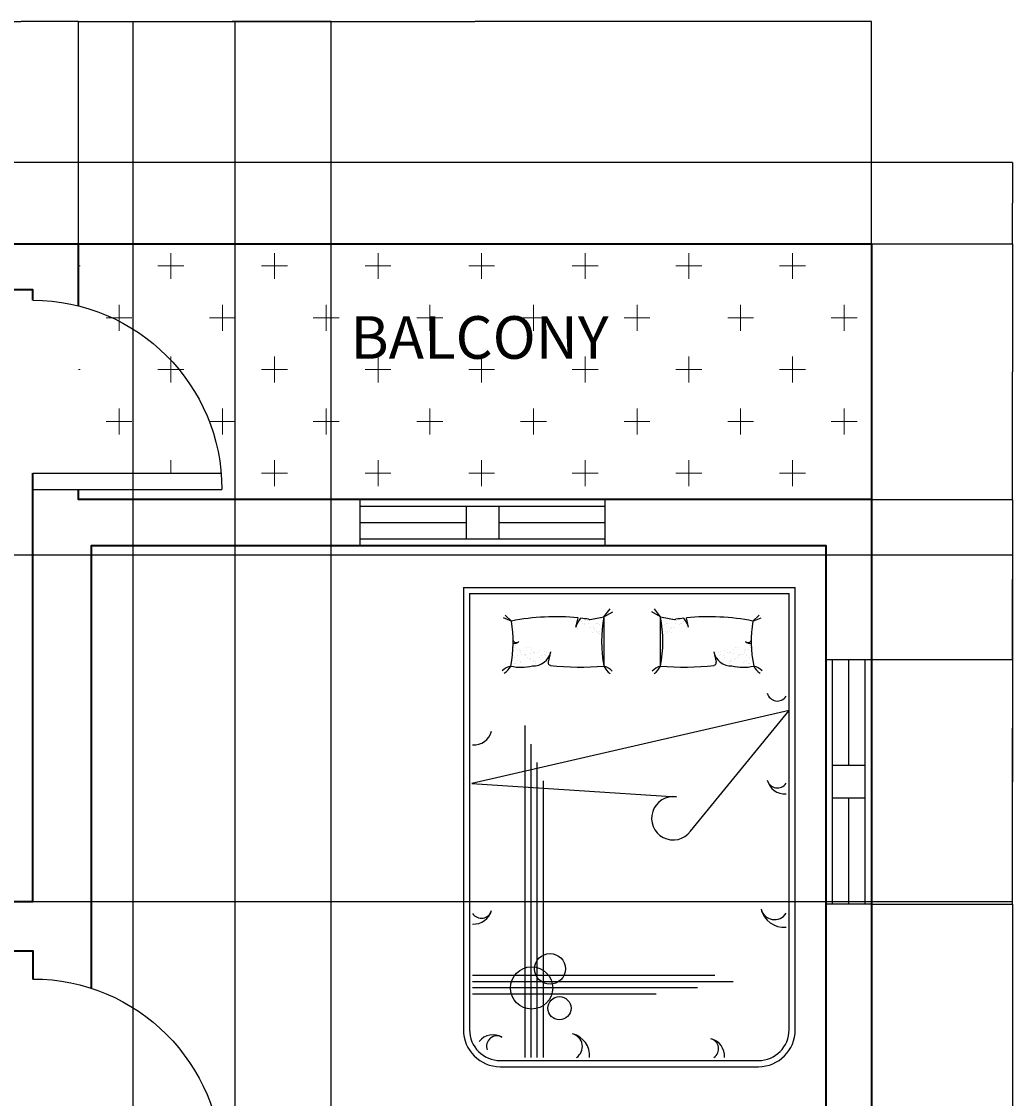
# Model space of a CAD drawing. Units: millimetres. Extents: x 19292 to 100733, y 12374 to 26974.
# Tile 22 of 24: x 52672 to 57530, y 18270 to 23551. Entities that reach past the tile are written whole.
import ezdxf

# ---------------------------------------------------------------- set-up
doc = ezdxf.new("R2010")
doc.units = ezdxf.units.MM
for name, color, linetype, lineweight in [('A-ANNO-DIMS', 2, 'Continuous', 18), ('A-AREA-IDEN', 3, 'Continuous', 25), ('A-DOOR', 4, 'Continuous', 25), ('A-FLOR-PATT', 252, 'Continuous', 13), ('A-FURN', 8, 'Continuous', 18), ('A-GLAZ', 3, 'Continuous', 25), ('A-WALL', 7, 'Continuous', 35)]:
    doc.layers.add(name, color=color, linetype=linetype, lineweight=lineweight)
doc.layers.add('FURNITURE', color=40, linetype='Continuous')
doc.layers.add('WINDOWS', color=50, linetype='Continuous')
doc.styles.get("Standard").update_dxf_attribs({"font": 'arial.ttf'})
doc.dimstyles.get("Standard").update_dxf_attribs({"dimtxt": 0.18, "dimasz": 0.18, "dimexe": 0.18, "dimexo": 0.0625, "dimgap": 0.09, "dimtad": 0, "dimtih": 1, "dimtoh": 1, "dimdec": 4, "dimzin": 0, "dimdsep": 46, "dimtxsty": 'Standard', "dimcen": 0.09, "dimadec": 0, "dimazin": 0, "dimtfac": 1, "dimtdec": 4, "dimtofl": 0, "dimtmove": 0, "dimatfit": 3, "dimfxl": 1, "dimtolj": 1, "dimtzin": 0, "dimarcsym": 0})

# ---------------------------------------------------------------- blocks, each defined once
blk = doc.blocks.new('WW')
at = {"layer": 'WINDOWS'}
for p, q in [((-5183.9, -4940.9), (-3983.9, -4940.9)), ((-4663.9, -4940.9), (-4663.9, -5100.9)), ((-4503.9, -4940.9), (-4503.9, -5100.9)), ((-4503.9, -4940.9), (-4503.9, -5100.9)), ((-5183.9, -5020.9), (-4663.9, -5020.9)), ((-4503.9, -5020.9), (-3983.9, -5020.9)), ((-5183.9, -5100.9), (-3983.9, -5100.9))]:
    blk.add_line(p, q, dxfattribs=at)
for points in [[(-5183.9, -5133.4), (-5183.9, -4908.4)], [(-3983.9, -4908.4), (-3983.9, -5133.4)]]:
    blk.add_lwpolyline(points, dxfattribs=at)
blk = doc.blocks.new('DBED-4FT6')
at = {"layer": 'FURNITURE'}
for p, q in [((-27, 0), (-27, -72)), ((-27, 0), (27, 0)), ((27, -72), (27, 0)), ((-26, -1), (-26, -72)), ((-26, -1), (26, -1)), ((26, -72), (26, -1)), ((-4.13, -4.82), (-3.14, -3.5)), ((5.06, -4.82), (4.07, -3.5)), ((-19.18, -5.49), (-20.5, -4.97)), ((-19.18, -5.49), (-20.21, -4.5)), ((-8.71, -6.49), (-8.35, -4.95)), ((-7.52, -5.09), (-7.52, -5.09)), ((-7.37, -5.22), (-7.37, -5.22)), ((-5.67, -5.22), (-5.67, -5.22)), ((-4.58, -5.08), (-4.58, -5.08)), ((-4.25, -5.03), (-4.25, -5.03)), ((-4.13, -4.82), (-2.71, -4)), ((5.06, -4.82), (3.64, -4)), ((5.18, -5.03), (5.18, -5.03)), ((5.51, -5.08), (5.51, -5.08)), ((6.6, -5.22), (6.6, -5.22)), ((8.29, -5.22), (8.29, -5.22)), ((8.44, -5.09), (8.44, -5.09)), ((9.64, -6.49), (9.28, -4.95)), ((20.11, -5.49), (21.13, -4.5)), ((20.11, -5.49), (21.43, -4.97)), ((-8.41, -6.64), (-8.41, -6.64)), ((-8.24, -5.56), (-8.24, -5.56)), ((-7.82, -5.51), (-7.82, -5.51)), ((-7.61, -5.81), (-7.61, -5.81)), ((-7.37, -5.85), (-7.37, -5.85)), ((-7.27, -6.02), (-7.27, -6.02)), ((-6.74, -5.36), (-6.74, -5.36)), ((-6.57, -5.95), (-6.57, -5.95)), ((-6.25, -6.56), (-6.25, -6.56)), ((-6.09, -5.28), (-6.09, -5.28)), ((-5.88, -6.59), (-5.88, -6.59)), ((-5.73, -6.73), (-5.73, -6.73)), ((-5.28, -5.82), (-5.28, -5.82)), ((-5.12, -5.81), (-5.12, -5.81)), ((-4.78, -6.02), (-4.78, -6.02)), ((5.71, -6.02), (5.71, -6.02)), ((6.05, -5.81), (6.05, -5.81)), ((6.21, -5.82), (6.21, -5.82)), ((6.65, -6.73), (6.65, -6.73)), ((6.8, -6.59), (6.8, -6.59)), ((7.01, -5.28), (7.01, -5.28)), ((7.17, -6.56), (7.17, -6.56)), ((7.5, -5.95), (7.5, -5.95)), ((7.66, -5.36), (7.66, -5.36)), ((8.2, -6.02), (8.2, -6.02)), ((8.3, -5.85), (8.3, -5.85)), ((8.54, -5.81), (8.54, -5.81)), ((8.75, -5.51), (8.75, -5.51)), ((9.17, -5.56), (9.17, -5.56)), ((9.33, -6.64), (9.33, -6.64)), ((-6, -7.34), (-6, -7.34)), ((-5.69, -7.03), (-5.69, -7.03)), ((-5.35, -7.25), (-5.35, -7.25)), ((-5.23, -7.36), (-5.23, -7.36)), ((-4.93, -7.2), (-4.93, -7.2)), ((-4.93, -7.46), (-4.93, -7.46)), ((5.86, -7.2), (5.86, -7.2)), ((5.86, -7.46), (5.86, -7.46)), ((6.16, -7.36), (6.16, -7.36)), ((6.27, -7.25), (6.27, -7.25)), ((6.61, -7.03), (6.61, -7.03)), ((6.92, -7.34), (6.92, -7.34)), ((-18.78, -9.84), (-18.78, -9.84)), ((-18.75, -9.83), (-18.75, -9.83)), ((-18.6, -9.46), (-18.6, -9.46)), ((-18.44, -10.05), (-18.44, -10.05)), ((-17.9, -10.1), (-17.9, -10.1)), ((-17.75, -10.24), (-17.75, -10.24)), ((-16.7, -9.84), (-16.7, -9.84)), ((-16.28, -9.83), (-16.28, -9.83)), ((-15.95, -10.05), (-15.95, -10.05)), ((-14.55, -10.26), (-14.55, -10.26)), ((-13.87, -10.45), (-13.87, -10.45)), ((-12.81, -10.5), (-13.21, -12.2)), ((13.73, -10.5), (14.13, -12.2)), ((14.8, -10.45), (14.8, -10.45)), ((15.48, -10.26), (15.48, -10.26)), ((16.87, -10.05), (16.87, -10.05)), ((17.21, -9.83), (17.21, -9.83)), ((17.63, -9.84), (17.63, -9.84)), ((18.68, -10.24), (18.68, -10.24)), ((18.83, -10.1), (18.83, -10.1)), ((19.36, -10.05), (19.36, -10.05)), ((19.52, -9.46), (19.52, -9.46)), ((19.67, -9.83), (19.67, -9.83)), ((19.7, -9.84), (19.7, -9.84)), ((-18.7, -11.37), (-18.7, -11.37)), ((-18.18, -11.01), (-18.18, -11.01)), ((-18.13, -11.84), (-18.13, -11.84)), ((-17.79, -12.06), (-17.79, -12.06)), ((-17.73, -10.63), (-17.73, -10.63)), ((-17.68, -12.17), (-17.68, -12.17)), ((-17.53, -10.93), (-17.53, -10.93)), ((-17.11, -10.87), (-17.11, -10.87)), ((-16.96, -10.97), (-16.96, -10.97)), ((-16.85, -11.06), (-16.85, -11.06)), ((-16.65, -11.38), (-16.65, -11.38)), ((-16.26, -11.6), (-16.26, -11.6)), ((-16.11, -11.74), (-16.11, -11.74)), ((-16.03, -10.73), (-16.03, -10.73)), ((-15.64, -11.84), (-15.64, -11.84)), ((-15.57, -10.56), (-15.57, -10.56)), ((-15.52, -12.1), (-15.52, -12.1)), ((-15.38, -10.64), (-15.38, -10.64)), ((-15.3, -12.05), (-15.3, -12.05)), ((-14.96, -10.59), (-14.96, -10.59)), ((-14.56, -11.36), (-14.56, -11.36)), ((-14.36, -11.06), (-14.36, -11.06)), ((-13.86, -10.9), (-13.86, -10.9)), ((-13.71, -11.04), (-13.71, -11.04)), ((-13.52, -10.57), (-13.52, -10.57)), ((14.45, -10.57), (14.45, -10.57)), ((14.63, -11.04), (14.63, -11.04)), ((14.78, -10.9), (14.78, -10.9)), ((15.29, -11.06), (15.29, -11.06)), ((15.48, -11.36), (15.48, -11.36)), ((15.89, -10.59), (15.89, -10.59)), ((16.23, -12.05), (16.23, -12.05)), ((16.3, -10.64), (16.3, -10.64)), ((16.45, -12.1), (16.45, -12.1)), ((16.5, -10.56), (16.5, -10.56)), ((16.56, -11.84), (16.56, -11.84)), ((16.95, -10.73), (16.95, -10.73)), ((17.04, -11.74), (17.04, -11.74)), ((17.19, -11.6), (17.19, -11.6)), ((17.58, -11.38), (17.58, -11.38)), ((17.78, -11.06), (17.78, -11.06)), ((17.88, -10.97), (17.88, -10.97)), ((18.04, -10.87), (18.04, -10.87)), ((18.46, -10.93), (18.46, -10.93)), ((18.61, -12.17), (18.61, -12.17)), ((18.66, -10.63), (18.66, -10.63)), ((18.72, -12.06), (18.72, -12.06)), ((19.06, -11.84), (19.06, -11.84)), ((19.11, -11.01), (19.11, -11.01)), ((19.62, -11.37), (19.62, -11.37)), ((-18.67, -12.31), (-18.67, -12.31)), ((-18.65, -12.91), (-18.65, -12.91)), ((-18.52, -12.44), (-18.52, -12.44)), ((-17.44, -12.99), (-17.44, -12.99)), ((-16.79, -12.9), (-16.79, -12.9)), ((-16.6, -12.92), (-16.6, -12.92)), ((-16.38, -12.85), (-16.38, -12.85)), ((-15.32, -12.47), (-15.32, -12.47)), ((-15.29, -12.7), (-15.29, -12.7)), ((16.22, -12.7), (16.22, -12.7)), ((16.24, -12.47), (16.24, -12.47)), ((17.3, -12.85), (17.3, -12.85)), ((17.53, -12.92), (17.53, -12.92)), ((17.72, -12.9), (17.72, -12.9)), ((18.37, -12.99), (18.37, -12.99)), ((19.44, -12.44), (19.44, -12.44)), ((19.57, -12.91), (19.57, -12.91)), ((19.59, -12.31), (19.59, -12.31)), ((26, -20.04), (-25.63, -31.9)), ((9.97, -39.68), (26, -20.04)), ((-16.98, -76.5), (-16.98, -22.5)), ((-15.98, -76.5), (-15.98, -25.5)), ((-14.98, -76.5), (-14.98, -28.5)), ((-13.98, -76.5), (-13.98, -31.5)), ((-25.63, -31.9), (7.69, -34.11)), ((13.92, -63.19), (-25.5, -63.19)), ((16.88, -64.19), (-25.5, -64.19)), ((11.1, -65.19), (-25.5, -65.19)), ((4.38, -66.19), (-25.5, -66.19)), ((-21, -77), (21, -77)), ((-21, -78), (21, -78))]:
    blk.add_line(p, q, dxfattribs=at)
for centre, radius in [((-12.91, -62.08), 2.5), ((-15.91, -65.19), 3.44), ((-11.37, -68.48), 1.88)]:
    blk.add_circle(centre, radius, dxfattribs=at)
for centre, radius, start, end in [((-11.96, -41.82), 37.04, 84.4029, 101.2371), ((-4.83, -7.61), 4.05, 139.9098, 163.9756), ((-11.52, -33.35), 28.57, 80.1409, 82.7554), ((-6.49, -4.41), 0.8, 260.1409, 276.0318), ((-67.64, 360.61), 370.91, 279.5022, 279.8589), ((15.67, -8.82), 20.2, 168.5788, 191.4212), ((15.67, -8.82), 20.2, 168.5788, 191.4212), ((42751.26, -8.82), 42755.4, 179.99464, 180.00536), ((-14.74, -8.82), 20.2, 348.5788, 11.4212), ((-42750.34, -8.82), 42755.4, 359.99464, 0.00536), ((-14.74, -8.82), 20.2, 348.5788, 11.4212), ((68.57, 360.61), 370.91, 260.1411, 260.4978), ((7.42, -4.41), 0.8, 263.9682, 279.8591), ((12.45, -33.35), 28.57, 97.2446, 99.8591), ((5.75, -7.61), 4.05, 16.0244, 40.0902), ((12.89, -41.82), 37.04, 78.7629, 95.5971), ((-39.11, -8.82), 20.2, 348.607, 9.4917), ((40.03, -8.82), 20.2, 170.5083, 191.393), ((-18.4, -8.45), 0.546, 201.8041, 319.1334), ((19.33, -8.45), 0.546, 220.8666, 338.1959), ((-18.63, -8.36), 0.782, 249.4969, 325.7978), ((-15.61, -9.92), 2.87, 266.7825, 348.1719), ((16.54, -9.92), 2.87, 191.8281, 273.2175), ((19.56, -8.36), 0.782, 214.2022, 290.5031), ((-12.82, -12.29), 0.4, 166.7873, 262.877), ((13.74, -12.29), 0.4, 277.123, 13.2127), ((-18.78, -15.36), 2.61, 101.6935, 136.5635), ((-21.65, -11.66), 2.61, 299.1485, 334.0185), ((-17.6, -5.62), 7.39, 256.6499, 284.2856), ((-7.85, 31.23), 44.21, 263.4826, 274.8199), ((-1.73, -11.81), 2.61, 202.7243, 237.5943), ((-4.81, -15.34), 2.61, 40.1792, 75.0493), ((5.73, -15.34), 2.61, 104.9507, 139.8208), ((2.65, -11.81), 2.61, 302.4057, 337.2757), ((8.78, 31.23), 44.21, 265.1801, 276.5174), ((18.52, -5.62), 7.39, 255.7144, 283.3501), ((19.7, -15.36), 2.61, 43.4365, 78.3065), ((22.58, -11.66), 2.61, 205.9815, 240.8515), ((24.08, -16.81), 1.69, 194.4515, 326.9106), ((-25.29, -22.71), 2.93, 265.8594, 345.9527), ((24.08, -30.96), 1.69, 194.4515, 326.9106), ((25.29, -30.67), 2.93, 194.0473, 274.1406), ((7.14, -37.58), 3.52, 81.0159, 323.3832), ((-25.29, -51.86), 2.93, 265.8594, 345.9527), ((-24.08, -52.15), 1.69, 213.0894, 345.5485), ((23.61, -51.81), 2.26, 194.4515, 326.9106), ((25.22, -51.42), 3.91, 194.0473, 274.1406), ((-21, -72), 6, 180, 270), ((-21, -72), 5, 180, 270), ((-22.19, -75.74), 2.93, 59.0473, 140.6217), ((-21.54, -74.68), 1.69, 59.4515, 200.6983), ((-9.76, -74.73), 2.12, 303.0894, 75.5485), ((-10.12, -76.24), 3.67, 355.8594, 75.9527), ((12.55, -76.29), 2.93, 355.8594, 75.9527), ((12.84, -75.08), 1.69, 303.0894, 75.5485), ((21, -72), 5, 270, 0), ((21, -72), 6, 270, 0)]:
    blk.add_arc(centre, radius, start, end, dxfattribs=at)
blk = doc.blocks.new('DOOR-SWING-900')
blk.add_line((927.7, 927.7), (927.7, 0))
blk.add_arc((927.7, 927.7), 927.7, 180, 270)
blk = doc.blocks.new('*D98')
at = {"layer": 'A-ANNO-DIMS', "color": 0, "lineweight": -2, "transparency": 16777216}
for p, q in [((52386.5, 22460.8), (52386.5, 23550.9)), ((52386.7, 23550.7), (52668.7, 23550.7)), ((52951.3, 23550.7), (52669.3, 23550.7)), ((52951.5, 22460.8), (52951.5, 23550.9))]:
    blk.add_line(p, q, dxfattribs=at)
at = {"layer": 'A-ANNO-DIMS', "color": 0, "transparency": 16777216}
for points in [[(52386.7, 23550.8), (52386.7, 23550.7), (52386.5, 23550.7)], [(52951.3, 23550.8), (52951.3, 23550.7), (52951.5, 23550.7)]]:
    blk.add_solid(points, dxfattribs=at)
at = {"layer": 'Defpoints', "color": 0, "transparency": 16777216}
for p in [(52951.5, 23550.7), (52386.5, 22460.7), (52951.5, 22460.7)]:
    blk.add_point(p, dxfattribs=at)
at = {"layer": 'A-ANNO-DIMS', "color": 0, "transparency": 16777216, "insert": (52669, 23550.7), "char_height": 0.18, "attachment_point": 5}
blk.add_mtext('\\A1;565', dxfattribs=at)
blk = doc.blocks.new('*D99')
at = {"layer": 'A-ANNO-DIMS', "color": 0, "lineweight": -2, "transparency": 16777216}
for p, q in [((52951.5, 22460.8), (52951.5, 23550.9)), ((52951.7, 23550.7), (54895, 23550.7)), ((56839, 23550.7), (54895.7, 23550.7)), ((56839.2, 22460.8), (56839.2, 23550.9))]:
    blk.add_line(p, q, dxfattribs=at)
at = {"layer": 'A-ANNO-DIMS', "color": 0, "transparency": 16777216}
for points in [[(52951.7, 23550.8), (52951.7, 23550.7), (52951.5, 23550.7)], [(56839, 23550.8), (56839, 23550.7), (56839.2, 23550.7)]]:
    blk.add_solid(points, dxfattribs=at)
at = {"layer": 'Defpoints', "color": 0, "transparency": 16777216}
for p in [(56839.2, 23550.7), (52951.5, 22460.7), (56839.2, 22460.7)]:
    blk.add_point(p, dxfattribs=at)
at = {"layer": 'A-ANNO-DIMS', "color": 0, "transparency": 16777216, "insert": (54895.3, 23550.7), "char_height": 0.18, "attachment_point": 5}
blk.add_mtext('\\A1;3888', dxfattribs=at)
blk = doc.blocks.new('*D102')
at = {"layer": 'A-ANNO-DIMS', "color": 0, "lineweight": -2, "transparency": 16777216}
for p, q in [((43614.1, 20935.7), (57530.2, 20935.7)), ((57530, 20935.5), (57530, 20085.9)), ((57530, 19235.9), (57530, 20085.5)), ((43614.1, 19235.7), (57530.2, 19235.7))]:
    blk.add_line(p, q, dxfattribs=at)
at = {"layer": 'A-ANNO-DIMS', "color": 0, "transparency": 16777216}
for points in [[(57530, 20935.5), (57530.1, 20935.5), (57530, 20935.7)], [(57530, 19235.9), (57530.1, 19235.9), (57530, 19235.7)]]:
    blk.add_solid(points, dxfattribs=at)
at = {"layer": 'Defpoints', "color": 0, "transparency": 16777216}
for p in [(43614, 20935.7), (43614, 19235.7), (57530, 19235.7)]:
    blk.add_point(p, dxfattribs=at)
at = {"layer": 'A-ANNO-DIMS', "color": 0, "transparency": 16777216, "insert": (57530, 20085.7), "char_height": 0.18, "attachment_point": 5}
blk.add_mtext('\\A1;1700', dxfattribs=at)
blk = doc.blocks.new('*D107')
at = {"layer": 'A-ANNO-DIMS', "color": 0, "lineweight": -2, "transparency": 16777216}
for p, q in [((56839.6, 19223.2), (57530.2, 19223.2)), ((57530, 19223), (57530, 17604.7)), ((57530, 15985.9), (57530, 17604.3)), ((56840.1, 15985.7), (57530.2, 15985.7))]:
    blk.add_line(p, q, dxfattribs=at)
at = {"layer": 'A-ANNO-DIMS', "color": 0, "transparency": 16777216}
for points in [[(57530, 19223), (57530.1, 19223), (57530, 19223.2)], [(57530, 15985.9), (57530.1, 15985.9), (57530, 15985.7)]]:
    blk.add_solid(points, dxfattribs=at)
at = {"layer": 'Defpoints', "color": 0, "transparency": 16777216}
for p in [(56839.5, 19223.2), (57530, 19223.2), (56840, 15985.7)]:
    blk.add_point(p, dxfattribs=at)
at = {"layer": 'A-ANNO-DIMS', "color": 0, "transparency": 16777216, "insert": (57530, 17604.5), "char_height": 0.18, "attachment_point": 5}
blk.add_mtext('\\A1;3237.5', dxfattribs=at)
blk = doc.blocks.new('*D108')
at = {"layer": 'A-ANNO-DIMS', "color": 0, "lineweight": -2, "transparency": 16777216}
for p, q in [((56839.6, 20423.2), (57530.2, 20423.2)), ((57530, 20423), (57530, 19823.4)), ((57530, 19223.4), (57530, 19823)), ((56839.6, 19223.2), (57530.2, 19223.2))]:
    blk.add_line(p, q, dxfattribs=at)
at = {"layer": 'A-ANNO-DIMS', "color": 0, "transparency": 16777216}
for points in [[(57530, 20423), (57530.1, 20423), (57530, 20423.2)], [(57530, 19223.4), (57530.1, 19223.4), (57530, 19223.2)]]:
    blk.add_solid(points, dxfattribs=at)
at = {"layer": 'Defpoints', "color": 0, "transparency": 16777216}
for p in [(56839.5, 20423.2), (57530, 20423.2), (56839.5, 19223.2)]:
    blk.add_point(p, dxfattribs=at)
at = {"layer": 'A-ANNO-DIMS', "color": 0, "transparency": 16777216, "insert": (57530, 19823.2), "char_height": 0.18, "attachment_point": 5}
blk.add_mtext('\\A1;1200', dxfattribs=at)
blk = doc.blocks.new('*D109')
at = {"layer": 'A-ANNO-DIMS', "color": 0, "lineweight": -2, "transparency": 16777216}
for p, q in [((56839.3, 21206.4), (57530.2, 21206.4)), ((57530, 21206.2), (57530, 20815)), ((57530, 20423.4), (57530, 20814.6)), ((56839.6, 20423.2), (57530.2, 20423.2))]:
    blk.add_line(p, q, dxfattribs=at)
at = {"layer": 'A-ANNO-DIMS', "color": 0, "transparency": 16777216}
for points in [[(57530, 21206.2), (57530.1, 21206.2), (57530, 21206.4)], [(57530, 20423.4), (57530.1, 20423.4), (57530, 20423.2)]]:
    blk.add_solid(points, dxfattribs=at)
at = {"layer": 'Defpoints', "color": 0, "transparency": 16777216}
for p in [(56839.2, 21206.4), (57530, 21206.4), (56839.5, 20423.2)]:
    blk.add_point(p, dxfattribs=at)
at = {"layer": 'A-ANNO-DIMS', "color": 0, "transparency": 16777216, "insert": (57530, 20814.8), "char_height": 0.18, "attachment_point": 5}
blk.add_mtext('\\A1;783.2', dxfattribs=at)
blk = doc.blocks.new('*D110')
at = {"layer": 'A-ANNO-DIMS', "color": 0, "lineweight": -2, "transparency": 16777216}
for p, q in [((56839.3, 22460.7), (57530.2, 22460.7)), ((57530, 22460.5), (57530, 21833.7)), ((57530, 21206.6), (57530, 21833.4)), ((56839.3, 21206.4), (57530.2, 21206.4))]:
    blk.add_line(p, q, dxfattribs=at)
at = {"layer": 'A-ANNO-DIMS', "color": 0, "transparency": 16777216}
for points in [[(57530, 22460.5), (57530.1, 22460.5), (57530, 22460.7)], [(57530, 21206.6), (57530.1, 21206.6), (57530, 21206.4)]]:
    blk.add_solid(points, dxfattribs=at)
at = {"layer": 'Defpoints', "color": 0, "transparency": 16777216}
for p in [(56839.2, 22460.7), (57530, 22460.7), (56839.2, 21206.4)]:
    blk.add_point(p, dxfattribs=at)
at = {"layer": 'A-ANNO-DIMS', "color": 0, "transparency": 16777216, "insert": (57530, 21833.6), "char_height": 0.18, "attachment_point": 5}
blk.add_mtext('\\A1;1254.3', dxfattribs=at)
blk = doc.blocks.new('*D111')
at = {"layer": 'A-ANNO-DIMS', "color": 0, "lineweight": -2, "transparency": 16777216}
for p, q in [((49064.1, 22860.7), (57530.2, 22860.7)), ((57530, 22860.5), (57530, 22660.9)), ((57530, 22460.9), (57530, 22660.5)), ((56839.3, 22460.7), (57530.2, 22460.7))]:
    blk.add_line(p, q, dxfattribs=at)
at = {"layer": 'A-ANNO-DIMS', "color": 0, "transparency": 16777216}
for points in [[(57530, 22860.5), (57530.1, 22860.5), (57530, 22860.7)], [(57530, 22460.9), (57530.1, 22460.9), (57530, 22460.7)]]:
    blk.add_solid(points, dxfattribs=at)
at = {"layer": 'Defpoints', "color": 0, "transparency": 16777216}
for p in [(49064, 22860.7), (57530, 22860.7), (56839.2, 22460.7)]:
    blk.add_point(p, dxfattribs=at)
at = {"layer": 'A-ANNO-DIMS', "color": 0, "transparency": 16777216, "insert": (57530, 22660.7), "char_height": 0.18, "attachment_point": 5}
blk.add_mtext('\\A1;400', dxfattribs=at)
blk = doc.blocks.new('*D112')
at = {"layer": 'A-ANNO-DIMS', "color": 0, "lineweight": -2, "transparency": 16777216}
for p, q in [((43389, 22860.7), (43389, 12813.8)), ((56840, 15985.7), (56840, 12813.8)), ((43389.2, 12814), (50114.1, 12814)), ((56839.9, 12814), (50114.9, 12814))]:
    blk.add_line(p, q, dxfattribs=at)
at = {"layer": 'A-ANNO-DIMS', "color": 0, "transparency": 16777216}
for points in [[(43389.2, 12814), (43389.2, 12814), (43389, 12814)], [(56839.9, 12814), (56839.9, 12814), (56840, 12814)]]:
    blk.add_solid(points, dxfattribs=at)
at = {"layer": 'Defpoints', "color": 0, "transparency": 16777216}
for p in [(43389, 22860.7), (56840, 15985.7), (56840, 12814)]:
    blk.add_point(p, dxfattribs=at)
at = {"layer": 'A-ANNO-DIMS', "color": 0, "transparency": 16777216, "insert": (50114.5, 12814), "char_height": 0.18, "attachment_point": 5}
blk.add_mtext('\\A1;13451', dxfattribs=at)
blk = doc.blocks.new('*D117')
at = {"layer": 'A-ANNO-DIMS', "color": 0, "lineweight": -2, "transparency": 16777216}
for p, q in [((53718.5, 15131.5), (53718.5, 23550.9)), ((53718.6, 23550.7), (53953.6, 23550.7)), ((54189.3, 23550.7), (53954.4, 23550.7)), ((54189.5, 15131.5), (54189.5, 23550.9))]:
    blk.add_line(p, q, dxfattribs=at)
at = {"layer": 'A-ANNO-DIMS', "color": 0, "transparency": 16777216}
for points in [[(53718.6, 23550.8), (53718.6, 23550.7), (53718.5, 23550.7)], [(54189.3, 23550.8), (54189.3, 23550.7), (54189.5, 23550.7)]]:
    blk.add_solid(points, dxfattribs=at)
at = {"layer": 'Defpoints', "color": 0, "transparency": 16777216}
for p in [(54189.5, 23550.7), (53718.5, 15131.4), (54189.5, 15131.4)]:
    blk.add_point(p, dxfattribs=at)
at = {"layer": 'A-ANNO-DIMS', "color": 0, "transparency": 16777216, "insert": (53954, 23550.7), "char_height": 0.18, "attachment_point": 5}
blk.add_mtext('\\A1;471.1', dxfattribs=at)
blk = doc.blocks.new('*D120')
at = {"layer": 'A-ANNO-DIMS', "color": 0, "lineweight": -2, "transparency": 16777216}
for p, q in [((53219.5, 17056.5), (53219.5, 23550.9)), ((53219.7, 23550.7), (53704.2, 23550.7)), ((54189.3, 23550.7), (53704.8, 23550.7)), ((54189.5, 17056.5), (54189.5, 23550.9))]:
    blk.add_line(p, q, dxfattribs=at)
at = {"layer": 'A-ANNO-DIMS', "color": 0, "transparency": 16777216}
for points in [[(53219.7, 23550.8), (53219.7, 23550.7), (53219.5, 23550.7)], [(54189.3, 23550.8), (54189.3, 23550.7), (54189.5, 23550.7)]]:
    blk.add_solid(points, dxfattribs=at)
at = {"layer": 'Defpoints', "color": 0, "transparency": 16777216}
for p in [(54189.5, 23550.7), (53219.5, 17056.4), (54189.5, 17056.4)]:
    blk.add_point(p, dxfattribs=at)
at = {"layer": 'A-ANNO-DIMS', "color": 0, "transparency": 16777216, "insert": (53704.5, 23550.7), "char_height": 0.18, "attachment_point": 5}
blk.add_mtext('\\A1;970', dxfattribs=at)

msp = doc.modelspace()

# ---------------------------------------------------------------- hatches: boundary and pattern name
at = {"layer": 'A-FLOR-PATT'}
h = msp.add_hatch(dxfattribs=at)
h.set_pattern_fill('CROSS', color=256, scale=40)
h.paths.add_polyline_path([(56838.992, 22460.725), (52951.492, 22460.725), (52951.492, 22156.292, -0.3441564), (53654.209, 21256.287), (52951.492, 21256.287), (52951.492, 21206.403), (56839.196, 21206.403)])
h.paths.add_polyline_path([(52951.492, 22156.292), (52951.492, 21336.287), (53650.753, 21336.287, 0.32018853)], flags=17)
h.paths.add_polyline_path([(54230.787, 21839.662), (55733.419, 21839.662), (55733.419, 22163.868), (54230.787, 22163.868)], flags=24)

# ---------------------------------------------------------------- linework, layer by layer
at = {"layer": 'A-DOOR'}
msp.add_line((52726.51, 21336.287), (53650.753, 21336.287), dxfattribs=at)
at = {"layer": 'A-WALL'}
for points in [[(43388.992, 22860.725), (49063.992, 22860.725), (49063.992, 22460.725), (56838.992, 22460.725), (56840.043, 15985.725), (54414.519, 15985.331), (54414.519, 14906.403), (52089.658, 14906.403), (52089.658, 13543.993), (44043.674, 13543.993), (44026.778, 19012.695), (43388.992, 19010.725), (43388.992, 22860.725)], [(52951.492, 22156.292), (52951.492, 22460.725), (56839.196, 22460.725), (56839.196, 21206.403), (52951.492, 21206.403), (52951.492, 21256.287)], [(52726.51, 22183.986), (52726.51, 22235.725), (49001.51, 22235.725), (49001.51, 19235.725), (49053.956, 19235.725)], [(49949.607, 19235.725), (52726.51, 19235.725), (52726.51, 21336.287)], [(53014.796, 18809.957), (53014.796, 20981.403), (56614.796, 20981.403), (56614.796, 17731.403), (55228.574, 17731.403)], [(49981.654, 18993.993), (52726.51, 18993.993), (52726.51, 18855.887)]]:
    msp.add_lwpolyline(points, dxfattribs=at)

# ---------------------------------------------------------------- block references
at = {"layer": 'A-DOOR', "extrusion": (0, 0, -1), "zscale": -1, "rotation": 269.9999999999991}
for p in [(-53654.209, 22183.986), (-53654.209, 18855.887)]:
    msp.add_blockref('DOOR-SWING-900', p, dxfattribs=at)
at = {"layer": 'A-FURN', "xscale": 30.13269765108242, "yscale": 30.13269765108242, "zscale": 30.13269765108242}
msp.add_blockref('DBED-4FT6', (55652.036, 20776.357), dxfattribs=at)
at = {"layer": 'A-GLAZ'}
msp.add_blockref('WW', (59515.323, 26114.78), dxfattribs=at)
at = {"layer": 'A-GLAZ', "rotation": 270}
msp.add_blockref('WW', (61747.894, 15239.357), dxfattribs=at)

# ---------------------------------------------------------------- texts
at = {"layer": 'A-AREA-IDEN'}
msp.add_text('BALCONY', height=208.8711, dxfattribs=at).set_placement((54284.821, 21897.258))

# ---------------------------------------------------------------- dimensions: what is measured, and where the dimension line sits
at = {"layer": 'A-ANNO-DIMS'}
for base, p1, p2, override, picture, middle in [((52951.492, 23550.725), (52386.51, 22460.725), (52951.492, 22460.725), {"dimdec": 0, "dimlfac": 1, "dimrnd": 0, "dimzin": 0, "dimdsep": 46, "dimlunit": 2}, '*D98', (52669.001, 23550.725)), ((56839.196, 23550.725), (52951.492, 22460.725), (56839.196, 22460.725), {"dimdec": 0, "dimlfac": 1, "dimrnd": 0, "dimzin": 0, "dimdsep": 46, "dimlunit": 2}, '*D99', (54895.344, 23550.725)), ((54189.519, 23550.725), (53219.519, 17056.403), (54189.519, 17056.403), {"dimdec": 0, "dimlfac": 1, "dimrnd": 0, "dimzin": 0, "dimdsep": 46, "dimlunit": 2}, '*D120', (53704.519, 23550.725)), ((54189.519, 23550.725), (53718.457, 15131.403), (54189.519, 15131.403), {"dimdec": 1, "dimlfac": 1, "dimrnd": 0, "dimzin": 0, "dimdsep": 46, "dimlunit": 2}, '*D117', (53953.988, 23550.725)), ((56840.043, 12813.993), (43388.992, 22860.725), (56840.043, 15985.725), {"dimdec": 0, "dimlfac": 1, "dimrnd": 0, "dimzin": 0, "dimdsep": 46, "dimlunit": 2}, '*D112', (50114.517, 12813.993))]:
    dim = msp.add_linear_dim(base=base, p1=p1, p2=p2, dimstyle='Standard', override=override, dxfattribs=at)
    dim.commit()
    dim.dimension.update_dxf_attribs({"geometry": picture, "text_midpoint": middle})
for base, p1, p2, override, picture, middle in [((57530.043, 22860.725), (56839.196, 22460.725), (49063.992, 22860.725), {"dimdec": 0, "dimlfac": 1, "dimrnd": 0, "dimzin": 0, "dimdsep": 46, "dimlunit": 2}, '*D111', (57530.043, 22660.725)), ((57530.043, 22460.725), (56839.196, 21206.403), (56839.196, 22460.725), {"dimdec": 1, "dimlfac": 1, "dimrnd": 0, "dimzin": 0, "dimdsep": 46, "dimlunit": 2}, '*D110', (57530.043, 21833.564)), ((57530.043, 21206.403), (56839.517, 20423.225), (56839.196, 21206.403), {"dimdec": 1, "dimlfac": 1, "dimrnd": 0, "dimzin": 0, "dimdsep": 46, "dimlunit": 2}, '*D109', (57530.043, 20814.814)), ((57530.043, 19235.725), (43613.992, 20935.725), (43613.992, 19235.725), {"dimdec": 0, "dimlfac": 1, "dimrnd": 0, "dimzin": 0, "dimdsep": 46, "dimlunit": 2}, '*D102', (57530.043, 20085.725)), ((57530.043, 20423.225), (56839.517, 19223.225), (56839.517, 20423.225), {"dimdec": 0, "dimlfac": 1, "dimrnd": 0, "dimzin": 0, "dimdsep": 46, "dimlunit": 2}, '*D108', (57530.043, 19823.225)), ((57530.043, 19223.225), (56840.043, 15985.725), (56839.517, 19223.225), {"dimdec": 1, "dimlfac": 1, "dimrnd": 0, "dimzin": 0, "dimdsep": 46, "dimlunit": 2}, '*D107', (57530.043, 17604.475))]:
    dim = msp.add_linear_dim(base=base, p1=p1, p2=p2, angle=90, dimstyle='Standard', override=override, dxfattribs=at)
    dim.commit()
    dim.dimension.update_dxf_attribs({"geometry": picture, "text_midpoint": middle})

doc.saveas('drawing.dxf')
